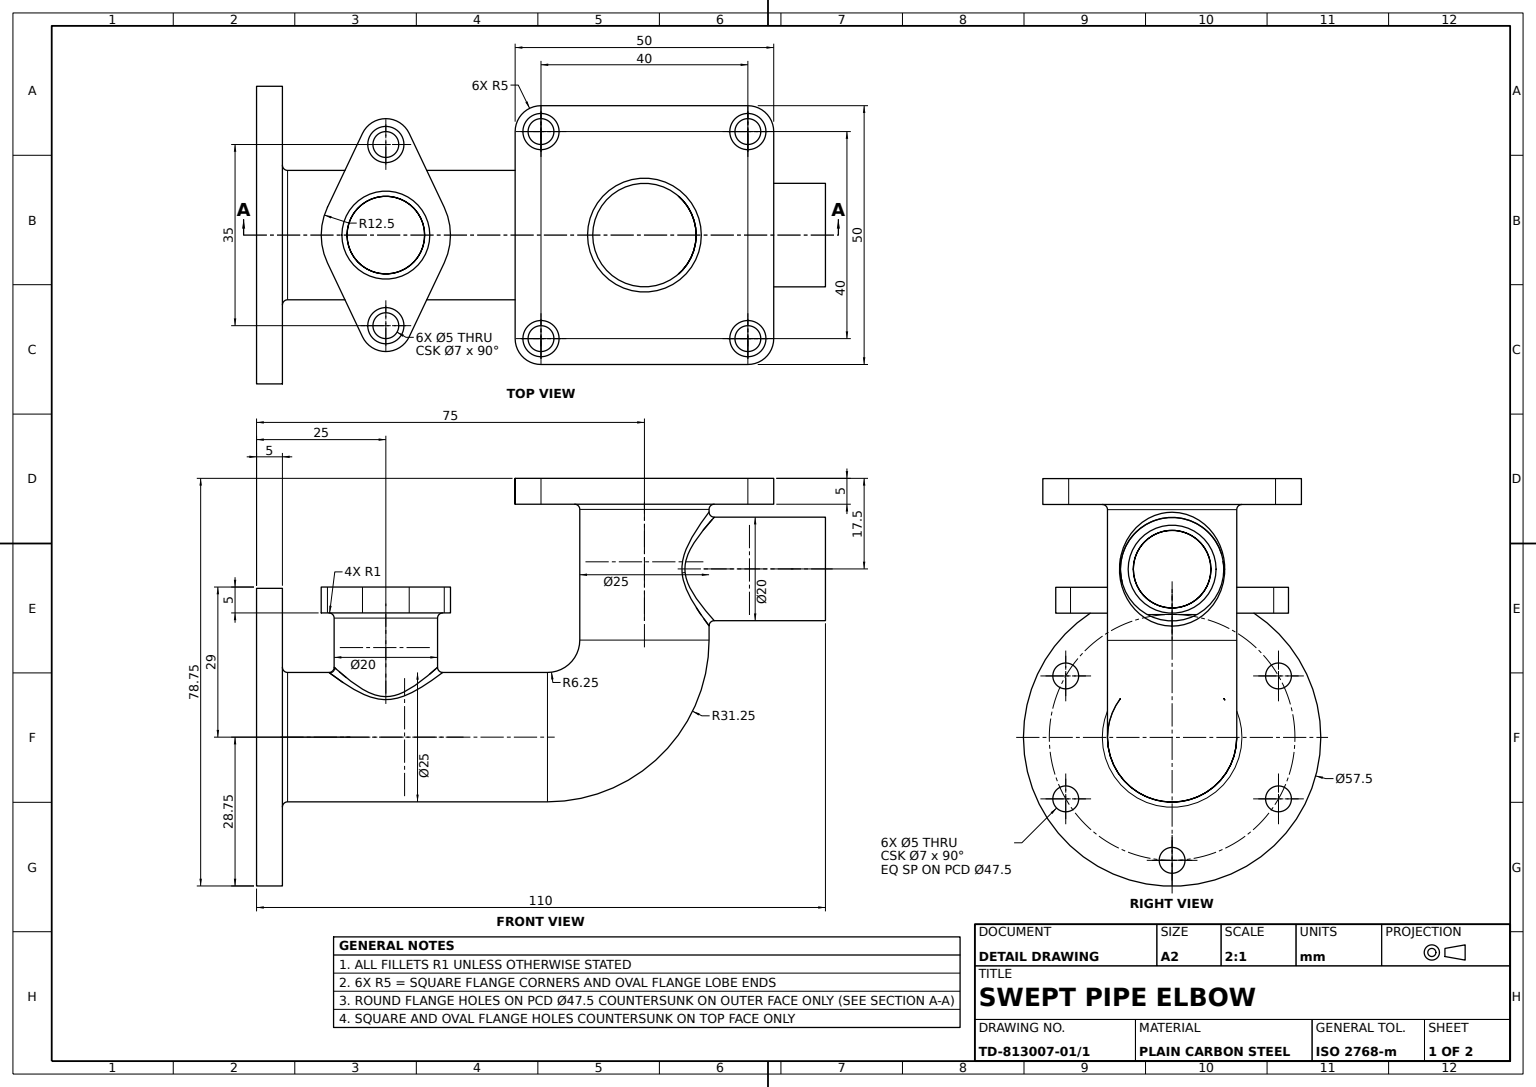
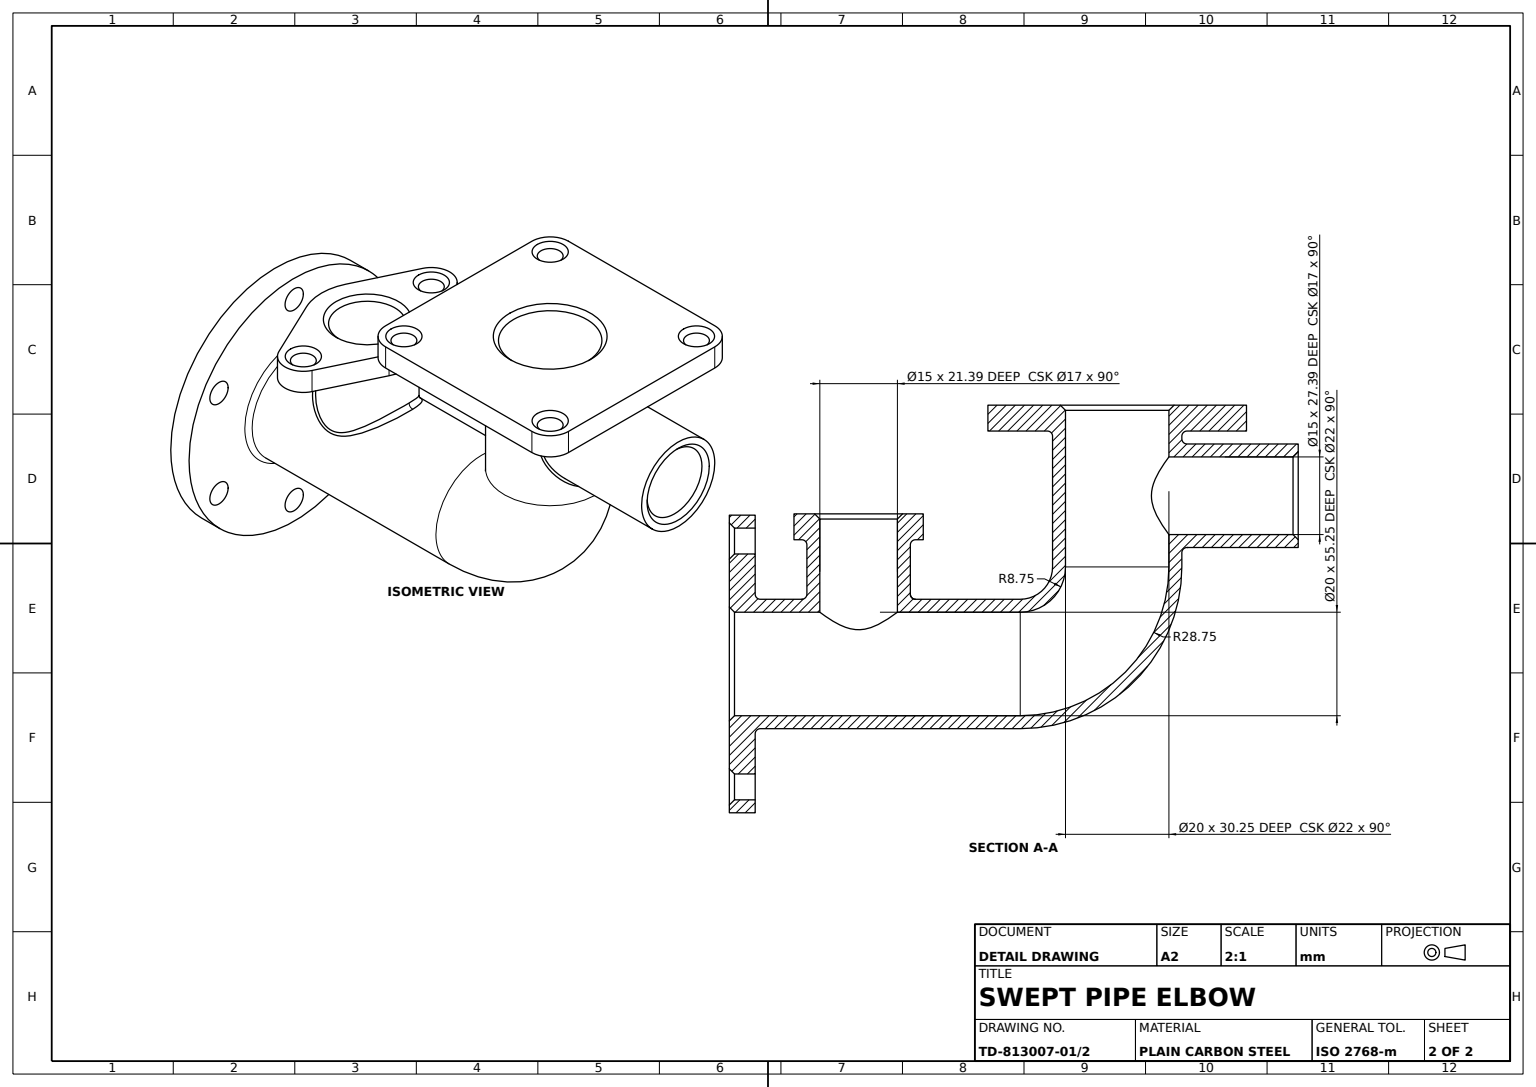
from build123d import *

# Parameters (mm, degrees)
ELBOW_PIPE_25_PROFILE_R        = 12.5
SIDE_BOSS_SKETCH_R             = 10
SIDE_BOSS_20_DEPTH             = 35
BRANCH_BOSS_SKETCH_R           = 10
BRANCH_BOSS_20_DEPTH           = 29
ROUND_FLANGE_SKETCH_R          = 28.75
ROUND_FLANGE_SKETCH_R_2        = 2.5
ROUND_FLANGE_57_5_6X_5_DEPTH   = 5
SQUARE_FLANGE_SKETCH_R         = 2.5
SQUARE_FLANGE_50X50_4X_5_DEPTH = 5
OVAL_FLANGE_SKETCH_R           = 2.5
OVAL_BRANCH_FLANGE_2X_5_DEPTH  = 5
ELBOW_BORE_20_PROFILE_R        = 10
BRANCH_BORE_15_REACH           = 129.521
BRANCH_BORE_15_END_RADIUS      = 10
BRANCH_BORE_SKETCH_R           = 7.5
SIDE_BOSS_BORE_15_REACH        = 126.204
SIDE_BOSS_BORE_15_END_RADIUS   = 10
SIDE_BOSS_BORE_SKETCH_R        = 7.5
ELBOW_BORE_CHAMFER_1MM_SIZE    = 1
EDGE_CHAMFERS_1MM_SIZE         = 1
EDGE_FILLETS_R1_R              = 1


with BuildPart() as part:
    # Elbow Pipe _25: sweep along a path in Elbow Path Sketch
    with BuildLine(Plane(origin=(0, 0, 0), x_dir=(0, 0, -1), z_dir=(1, 0, 0))) as elbow_pipe_25_path:
        Line((0, 0), (56.25, 0))
        ThreePointArc((56.25, 0), (69.508252147, 5.491747853), (75, 18.75))
        Line((75, 18.75), (75, 50))
    # Elbow Pipe _25 profile (on start of the path) → Elbow Pipe _25 (sweep)
    with BuildSketch(Plane(origin=(0, 0, 0), x_dir=(-1, 0, 0), z_dir=(0, 0, -1))):
        Circle(ELBOW_PIPE_25_PROFILE_R)
    sweep(path=elbow_pipe_25_path.line)

    # Side Boss Sketch → Side Boss _20 (add)
    with BuildSketch(Plane.XY.offset(-75)):
        with Locations((0, 32.5)):
            Circle(SIDE_BOSS_SKETCH_R)
    extrude(amount=-SIDE_BOSS_20_DEPTH)

    # Branch Boss Sketch → Branch Boss _20 (add)
    with BuildSketch(Plane(origin=(0, 0, 0), x_dir=(1, 0, 0), z_dir=(0, 1, 0))):
        with Locations(Location((0, 25, 0), (0, 0, 90))):
            Circle(BRANCH_BOSS_SKETCH_R)
    extrude(amount=BRANCH_BOSS_20_DEPTH)

    # Round Flange Sketch → Round Flange _57.5 6x_5 (add)
    with BuildSketch(Plane.XY):
        Circle(ROUND_FLANGE_SKETCH_R)
        with Locations((0, 23.75)):
            Circle(ROUND_FLANGE_SKETCH_R_2, mode=Mode.SUBTRACT)
        with Locations((20.56810334, 11.875)):
            Circle(ROUND_FLANGE_SKETCH_R_2, mode=Mode.SUBTRACT)
        with Locations((20.56810334, -11.875)):
            Circle(ROUND_FLANGE_SKETCH_R_2, mode=Mode.SUBTRACT)
        with Locations((0, -23.75)):
            Circle(ROUND_FLANGE_SKETCH_R_2, mode=Mode.SUBTRACT)
        with Locations((-20.56810334, -11.875)):
            Circle(ROUND_FLANGE_SKETCH_R_2, mode=Mode.SUBTRACT)
        with Locations((-20.56810334, 11.875)):
            Circle(ROUND_FLANGE_SKETCH_R_2, mode=Mode.SUBTRACT)
    extrude(amount=-ROUND_FLANGE_57_5_6X_5_DEPTH)

    # Square Flange Sketch → Square Flange 50x50 4x_5 (add)
    with BuildSketch(Plane(origin=(0, 50, 0), x_dir=(1, 0, 0), z_dir=(0, 1, 0))):
        with BuildLine():
            Line((-20, 100), (20, 100))
            ThreePointArc((20, 100), (23.535533906, 98.535533906), (25, 95))
            Line((25, 95), (25, 55))
            ThreePointArc((25, 55), (23.535533906, 51.464466094), (20, 50))
            Line((20, 50), (-20, 50))
            ThreePointArc((-20, 50), (-23.535533906, 51.464466094), (-25, 55))
            Line((-25, 55), (-25, 95))
            ThreePointArc((-25, 95), (-23.535533906, 98.535533906), (-20, 100))
        make_face()
        with Locations(Location((-20, 95, 0), (0, 0, 270))):
            Circle(SQUARE_FLANGE_SKETCH_R, mode=Mode.SUBTRACT)
        with Locations(Location((20, 95, 0), (0, 0, 270))):
            Circle(SQUARE_FLANGE_SKETCH_R, mode=Mode.SUBTRACT)
        with Locations(Location((20, 55, 0), (0, 0, 270))):
            Circle(SQUARE_FLANGE_SKETCH_R, mode=Mode.SUBTRACT)
        with Locations(Location((-20, 55, 0), (0, 0, 270))):
            Circle(SQUARE_FLANGE_SKETCH_R, mode=Mode.SUBTRACT)
    extrude(amount=-SQUARE_FLANGE_50X50_4X_5_DEPTH)

    # Oval Flange Sketch → Oval Branch Flange 2x_5 (add)
    with BuildSketch(Plane(origin=(0, 29, 0), x_dir=(1, 0, 0), z_dir=(0, 1, 0))):
        with BuildLine():
            Line((-19.642857143, 29.517539515), (-5.357142857, 36.293848786))
            ThreePointArc((-5.357142857, 36.293848786), (0, 37.5), (5.357142857, 36.293848786))
            Line((5.357142857, 36.293848786), (19.642857143, 29.517539515))
            ThreePointArc((19.642857143, 29.517539515), (22.5, 25), (19.642857143, 20.482460485))
            Line((19.642857143, 20.482460485), (5.357142857, 13.706151214))
            ThreePointArc((5.357142857, 13.706151214), (0, 12.5), (-5.357142857, 13.706151214))
            Line((-5.357142857, 13.706151214), (-19.642857143, 20.482460485))
            ThreePointArc((-19.642857143, 20.482460485), (-22.5, 25), (-19.642857143, 29.517539515))
        make_face()
        with Locations(Location((-17.5, 25, 0), (0, 0, 270))):
            Circle(OVAL_FLANGE_SKETCH_R, mode=Mode.SUBTRACT)
        with Locations(Location((17.5, 25, 0), (0, 0, 270))):
            Circle(OVAL_FLANGE_SKETCH_R, mode=Mode.SUBTRACT)
    extrude(amount=-OVAL_BRANCH_FLANGE_2X_5_DEPTH)

    # Elbow Bore _20: sweep along a path in Sketch1_2
    with BuildLine(Plane(origin=(0, 0, 0), x_dir=(0, 0, -1), z_dir=(1, 0, 0))) as elbow_bore_20_path:
        Line((0, 0), (56.25, 0))
        ThreePointArc((56.25, 0), (69.508252147, 5.491747853), (75, 18.75))
        Line((75, 18.75), (75, 50))
    # Elbow Bore _20 profile (on start of the path) → Elbow Bore _20 (sweep, cut)
    with BuildSketch(Plane(origin=(0, 0, 0), x_dir=(-1, 0, 0), z_dir=(0, 0, -1))):
        Circle(ELBOW_BORE_20_PROFILE_R)
    sweep(path=elbow_bore_20_path.line, mode=Mode.SUBTRACT)

    # Branch Bore _15: up to this cylinder (the profile starts outside it)
    branch_bore_15_end = Plane(origin=(0, 0, -25), z_dir=(0, 0, -1)) * Cylinder(BRANCH_BORE_15_END_RADIUS, 280.042, mode=Mode.PRIVATE)
    # Branch Bore Sketch → Branch Bore _15 (cut, up to the surface)
    with BuildSketch(Plane(origin=(0, 29, 0), x_dir=(1, 0, 0), z_dir=(0, 1, 0)), mode=Mode.PRIVATE) as branch_bore_15_sk1:
        with Locations(Location((0, 25, 0), (0, 0, 270))):
            Circle(BRANCH_BORE_SKETCH_R)
    branch_bore_15_tool1 = extrude(branch_bore_15_sk1.sketch, amount=-BRANCH_BORE_15_REACH, mode=Mode.PRIVATE) - branch_bore_15_end
    add(branch_bore_15_tool1.solids().sort_by_distance((0, 29, -25))[0], mode=Mode.SUBTRACT)

    # Side Boss Bore _15: up to this cylinder (the profile starts outside it)
    side_boss_bore_15_end = Plane(origin=(0, 32.5, -75), z_dir=(0, 1, 0)) * Cylinder(SIDE_BOSS_BORE_15_END_RADIUS, 273.408, mode=Mode.PRIVATE)
    # Side Boss Bore Sketch → Side Boss Bore _15 (cut, up to the surface)
    with BuildSketch(Plane(origin=(0, 0, -110), x_dir=(-1, 0, 0), z_dir=(0, 0, -1)), mode=Mode.PRIVATE) as side_boss_bore_15_sk1:
        with Locations((0, 32.5)):
            Circle(SIDE_BOSS_BORE_SKETCH_R)
    side_boss_bore_15_tool1 = extrude(side_boss_bore_15_sk1.sketch, amount=-SIDE_BOSS_BORE_15_REACH, mode=Mode.PRIVATE) - side_boss_bore_15_end
    add(side_boss_bore_15_tool1.solids().sort_by_distance((0, 32.5, -110))[0], mode=Mode.SUBTRACT)

    # Elbow Bore Chamfer 1mm
    elbow_bore_chamfer_1mm_edges = [part.edges().sort_by_distance(p)[0] for p in [
        (10, 0, 0),
    ]]
    chamfer(elbow_bore_chamfer_1mm_edges, length=ELBOW_BORE_CHAMFER_1MM_SIZE)

    # Edge Chamfers 1mm
    edge_chamfers_1mm_edges = [part.edges().sort_by_distance(p)[0] for p in [
        (0, 29, -32.5),
        (7.5, 32.5, -110),
        (-2.5, 23.75, 0),
        (18.06810334, 11.875, 0),
        (18.06810334, -11.875, 0),
        (-2.5, -23.75, 0),
        (-23.06810334, -11.875, 0),
        (-23.06810334, 11.875, 0),
        (-20, 50, -97.5),
        (20, 50, -97.5),
        (20, 50, -57.5),
        (-20, 50, -57.5),
        (-17.5, 29, -27.5),
        (17.5, 29, -27.5),
        (10, 50, -75),
    ]]
    chamfer(edge_chamfers_1mm_edges, length=EDGE_CHAMFERS_1MM_SIZE)

    # Edge Fillets R1
    edge_fillets_r1_edges = [part.edges().sort_by_distance(p)[0] for p in [
        (-10, 32.5, -82.5),
        (-2e-09, 12.50000001, -14.999999996),
        (12.5, 0, -5),
        (12.5, 45, -75),
        (0, 24, -15),
    ]]
    fillet(edge_fillets_r1_edges, radius=EDGE_FILLETS_R1_R)


solid = part.part
